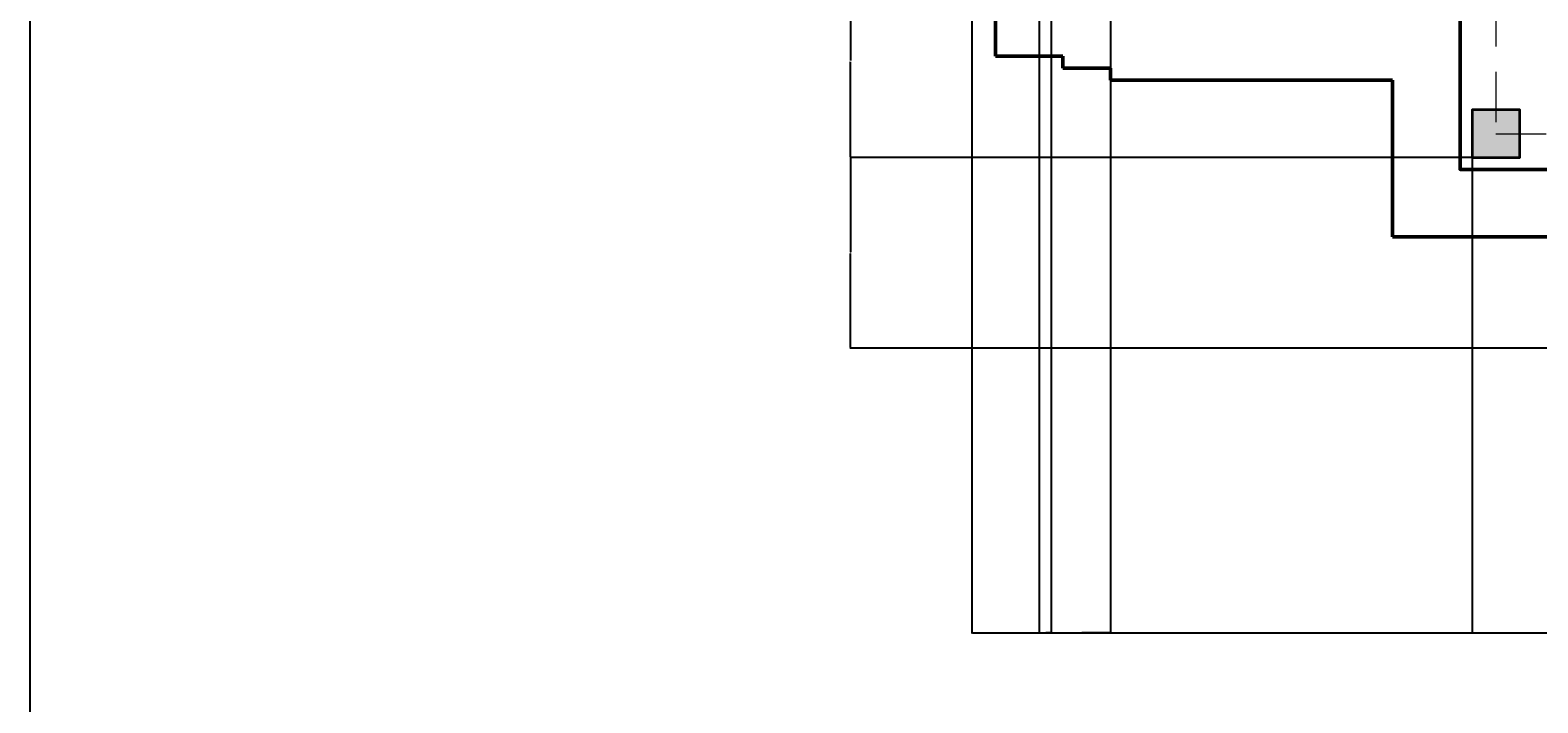
# Model space of a CAD drawing. Units: inches. Extents: x 386 to 107067, y -7 to 96314.
# Tile 3 of 10: x 386 to 766, y 855 to 1024. Entities that reach past the tile are written whole.
import ezdxf

# ---------------------------------------------------------------- set-up
doc = ezdxf.new("R2010")
doc.units = ezdxf.units.IN
doc.linetypes.add('DASHED', pattern=[19.05, 12.7, -6.35])
for name, color, linetype, lineweight in [('A-ANNO-DIMS', 2, 'Continuous', 18), ('A-COLS', 1, 'Continuous', 35), ('A-ELEV', 7, 'Continuous', 25), ('A-FLOR-OVHD', 8, 'DASHED', 18), ('A-WALL', 7, 'Continuous', 50)]:
    doc.layers.add(name, color=color, linetype=linetype, lineweight=lineweight)
doc.styles.get("Standard").update_dxf_attribs({"font": 'arial.ttf'})
doc.dimstyles.get("Standard").update_dxf_attribs({"dimtxt": 0.18, "dimasz": 0.18, "dimexe": 0.18, "dimexo": 0.0625, "dimgap": 0.09, "dimtad": 0, "dimtih": 1, "dimtoh": 1, "dimdec": 4, "dimzin": 0, "dimdsep": 46, "dimtxsty": 'Standard', "dimcen": 0.09, "dimadec": 0, "dimazin": 0, "dimtfac": 1, "dimtdec": 4, "dimtofl": 0, "dimtmove": 0, "dimatfit": 3, "dimfxl": 1, "dimtolj": 1, "dimtzin": 0, "dimarcsym": 0})

# ---------------------------------------------------------------- blocks, each defined once
blk = doc.blocks.new('COL-300')
h = blk.add_hatch(color=256)
h.dxf.hatch_style = 1
h.paths.add_polyline_path([(761.03, 1172.09), (749.03, 1172.09), (749.03, 1160.09), (761.03, 1160.09)])
blk.add_lwpolyline([(749.03, 1160.09), (761.03, 1160.09), (761.03, 1172.09), (749.03, 1172.09)], close=True)
blk = doc.blocks.new('*D8')
at = {"layer": 'A-ANNO-DIMS', "color": 0, "lineweight": -2, "transparency": 16777216}
for p, q in [((623.03, 1046.53), (623.03, 872.22)), ((1169.03, 1014.03), (1169.03, 872.22)), ((623.21, 872.4), (895.74, 872.4)), ((1168.85, 872.4), (896.31, 872.4))]:
    blk.add_line(p, q, dxfattribs=at)
at = {"layer": 'A-ANNO-DIMS', "color": 0, "transparency": 16777216}
for points in [[(623.21, 872.43), (623.21, 872.37), (623.03, 872.4)], [(1168.85, 872.43), (1168.85, 872.37), (1169.03, 872.4)]]:
    blk.add_solid(points, dxfattribs=at)
at = {"layer": 'Defpoints', "color": 0, "transparency": 16777216}
for p in [(623.03, 1046.59), (1169.03, 1014.09), (1169.03, 872.4)]:
    blk.add_point(p, dxfattribs=at)
at = {"layer": 'A-ANNO-DIMS', "color": 0, "transparency": 16777216, "insert": (896.03, 872.4), "char_height": 0.18, "attachment_point": 5}
blk.add_mtext('\\A1;546', dxfattribs=at)
blk = doc.blocks.new('*D27')
at = {"layer": 'A-ANNO-DIMS', "color": 0, "lineweight": -2, "transparency": 16777216}
for p, q in [((749.03, 992.03), (749.03, 872.22)), ((791.03, 992.03), (791.03, 872.22)), ((749.21, 872.4), (769.8, 872.4)), ((790.85, 872.4), (770.25, 872.4))]:
    blk.add_line(p, q, dxfattribs=at)
at = {"layer": 'A-ANNO-DIMS', "color": 0, "transparency": 16777216}
for points in [[(749.21, 872.43), (749.21, 872.37), (749.03, 872.4)], [(790.85, 872.43), (790.85, 872.37), (791.03, 872.4)]]:
    blk.add_solid(points, dxfattribs=at)
at = {"layer": 'Defpoints', "color": 0, "transparency": 16777216}
for p in [(749.03, 992.09), (791.03, 992.09), (791.03, 872.4)]:
    blk.add_point(p, dxfattribs=at)
at = {"layer": 'A-ANNO-DIMS', "color": 0, "transparency": 16777216, "insert": (770.03, 872.4), "char_height": 0.18, "attachment_point": 5}
blk.add_mtext('\\A1;42', dxfattribs=at)
blk = doc.blocks.new('*D31')
at = {"layer": 'A-ANNO-DIMS', "color": 0, "lineweight": -2, "transparency": 16777216}
for p, q in [((748.96, 992.09), (592.35, 992.09)), ((592.53, 991.91), (592.53, 968.27)), ((592.53, 944.27), (592.53, 967.91)), ((790.96, 944.09), (592.35, 944.09))]:
    blk.add_line(p, q, dxfattribs=at)
at = {"layer": 'A-ANNO-DIMS', "color": 0, "transparency": 16777216}
for points in [[(592.5, 991.91), (592.56, 991.91), (592.53, 992.09)], [(592.5, 944.27), (592.56, 944.27), (592.53, 944.09)]]:
    blk.add_solid(points, dxfattribs=at)
at = {"layer": 'Defpoints', "color": 0, "transparency": 16777216}
for p in [(592.53, 992.09), (749.03, 992.09), (791.03, 944.09)]:
    blk.add_point(p, dxfattribs=at)
at = {"layer": 'A-ANNO-DIMS', "color": 0, "transparency": 16777216, "insert": (592.53, 968.09), "char_height": 0.18, "attachment_point": 5}
blk.add_mtext('\\A1;48', dxfattribs=at)
blk = doc.blocks.new('*D32')
at = {"layer": 'A-ANNO-DIMS', "color": 0, "lineweight": -2, "transparency": 16777216}
for p, q in [((748.96, 1040.59), (592.35, 1040.59)), ((592.53, 1040.41), (592.53, 1016.52)), ((592.53, 992.27), (592.53, 1016.16)), ((748.96, 992.09), (592.35, 992.09))]:
    blk.add_line(p, q, dxfattribs=at)
at = {"layer": 'A-ANNO-DIMS', "color": 0, "transparency": 16777216}
for points in [[(592.5, 1040.41), (592.56, 1040.41), (592.53, 1040.59)], [(592.5, 992.27), (592.56, 992.27), (592.53, 992.09)]]:
    blk.add_solid(points, dxfattribs=at)
at = {"layer": 'Defpoints', "color": 0, "transparency": 16777216}
for p in [(592.53, 1040.59), (749.03, 1040.59), (749.03, 992.09)]:
    blk.add_point(p, dxfattribs=at)
at = {"layer": 'A-ANNO-DIMS', "color": 0, "transparency": 16777216, "insert": (592.53, 1016.34), "char_height": 0.18, "attachment_point": 5}
blk.add_mtext('\\A1;48.5', dxfattribs=at)
blk = doc.blocks.new('*D44')
at = {"layer": 'A-ANNO-DIMS', "color": 0, "lineweight": -2, "transparency": 16777216}
for p, q in [((640.03, 1064.28), (640.03, 872.22)), ((643.03, 1064.28), (643.03, 872.22)), ((640.21, 872.4), (641.38, 872.4)), ((642.85, 872.4), (641.67, 872.4))]:
    blk.add_line(p, q, dxfattribs=at)
at = {"layer": 'A-ANNO-DIMS', "color": 0, "transparency": 16777216}
for points in [[(640.21, 872.43), (640.21, 872.37), (640.03, 872.4)], [(642.85, 872.43), (642.85, 872.37), (643.03, 872.4)]]:
    blk.add_solid(points, dxfattribs=at)
at = {"layer": 'Defpoints', "color": 0, "transparency": 16777216}
for p in [(640.03, 1064.34), (643.03, 1064.34), (643.03, 872.4)]:
    blk.add_point(p, dxfattribs=at)
at = {"layer": 'A-ANNO-DIMS', "color": 0, "transparency": 16777216, "insert": (641.53, 872.4), "char_height": 0.18, "attachment_point": 5}
blk.add_mtext('\\A1;3', dxfattribs=at)
blk = doc.blocks.new('*D45')
at = {"layer": 'A-ANNO-DIMS', "color": 0, "lineweight": -2, "transparency": 16777216}
for p, q in [((643.03, 1046.53), (643.03, 872.22)), ((658.03, 1046.53), (658.03, 872.22)), ((643.21, 872.4), (650.31, 872.4)), ((657.85, 872.4), (650.74, 872.4))]:
    blk.add_line(p, q, dxfattribs=at)
at = {"layer": 'A-ANNO-DIMS', "color": 0, "transparency": 16777216}
for points in [[(643.21, 872.43), (643.21, 872.37), (643.03, 872.4)], [(657.85, 872.43), (657.85, 872.37), (658.03, 872.4)]]:
    blk.add_solid(points, dxfattribs=at)
at = {"layer": 'Defpoints', "color": 0, "transparency": 16777216}
for p in [(643.03, 1046.59), (658.03, 1046.59), (658.03, 872.4)]:
    blk.add_point(p, dxfattribs=at)
at = {"layer": 'A-ANNO-DIMS', "color": 0, "transparency": 16777216, "insert": (650.53, 872.4), "char_height": 0.18, "attachment_point": 5}
blk.add_mtext('\\A1;15', dxfattribs=at)

msp = doc.modelspace()

# ---------------------------------------------------------------- linework, layer by layer
at = {"layer": 'A-ELEV'}
msp.add_lwpolyline([(385.946, 1737.774), (1886.0535, 1737.774), (1886.0535, -7.0679), (385.946, -7.0679)], close=True, dxfattribs=at)
at = {"layer": 'A-FLOR-OVHD'}
msp.add_lwpolyline([(755.0252, 998.0919), (923.0252, 998.0919), (923.0252, 1166.0919), (755.0252, 1166.0919)], close=True, dxfattribs=at)
at = {"layer": 'A-WALL'}
for p, q in [((629.0252, 1031.5919), (629.0252, 1017.5919)), ((646.0252, 1017.5919), (646.0252, 1014.5919)), ((658.0252, 1014.5919), (658.0252, 1011.5919)), ((729.0252, 972.0919), (729.0252, 1011.5919))]:
    msp.add_line(p, q, dxfattribs=at)
for points in [[(788.0252, 1175.0919), (746.0252, 1175.0919), (746.0252, 989.0919), (788.0252, 989.0919)], [(629.0252, 1017.5919), (646.0252, 1017.5919)], [(646.0252, 1014.5919), (658.0252, 1014.5919)], [(658.0252, 1011.5919), (729.0252, 1011.5919)], [(729.0252, 972.0919), (771.0252, 972.0919)]]:
    msp.add_lwpolyline(points, dxfattribs=at)

# ---------------------------------------------------------------- block references
at = {"layer": 'A-COLS'}
msp.add_blockref('COL-300', (0, -168), dxfattribs=at)

# ---------------------------------------------------------------- dimensions: what is measured, and where the dimension line sits
at = {"layer": 'A-ANNO-DIMS'}
for base, p1, p2, picture, middle in [((643.0252, 872.3951), (640.0252, 1064.3399), (643.0252, 1064.3399), '*D44', (641.5252, 872.3951)), ((1169.0252, 872.3951), (623.0252, 1046.5919), (1169.0252, 1014.0919), '*D8', (896.0252, 872.3951)), ((658.0252, 872.3951), (643.0252, 1046.5919), (658.0252, 1046.5919), '*D45', (650.5252, 872.3951)), ((791.0252, 872.3951), (749.0252, 992.0919), (791.0252, 992.0919), '*D27', (770.0252, 872.3951))]:
    dim = msp.add_linear_dim(base=base, p1=p1, p2=p2, dimstyle='Standard', override={"dimdec": 0, "dimlfac": 1, "dimrnd": 0, "dimzin": 0, "dimdsep": 46, "dimlunit": 2}, dxfattribs=at)
    dim.commit()
    dim.dimension.update_dxf_attribs({"geometry": picture, "text_midpoint": middle})
for base, p1, p2, override, picture, middle in [((592.5252, 1040.5919), (749.0252, 992.0919), (749.0252, 1040.5919), {"dimdec": 1, "dimlfac": 1, "dimrnd": 0, "dimzin": 0, "dimdsep": 46, "dimlunit": 2}, '*D32', (592.5252, 1016.3419)), ((592.5252, 992.0919), (791.0252, 944.0919), (749.0252, 992.0919), {"dimdec": 0, "dimlfac": 1, "dimrnd": 0, "dimzin": 0, "dimdsep": 46, "dimlunit": 2}, '*D31', (592.5252, 968.0919))]:
    dim = msp.add_linear_dim(base=base, p1=p1, p2=p2, angle=90, dimstyle='Standard', override=override, dxfattribs=at)
    dim.commit()
    dim.dimension.update_dxf_attribs({"geometry": picture, "text_midpoint": middle})

doc.saveas('drawing.dxf')
